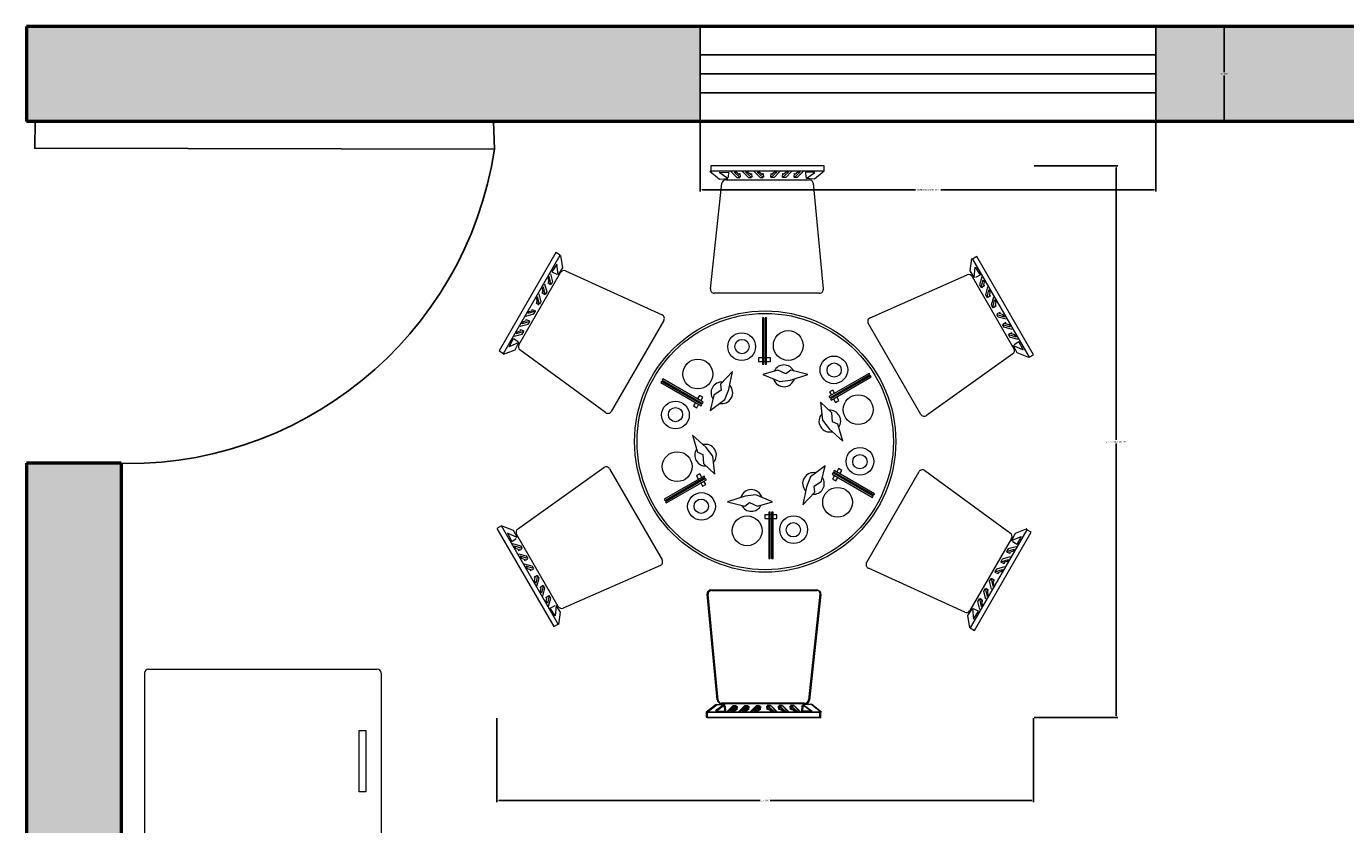
# Model space of a CAD drawing. Units: inches. Extents: x 1771 to 3025, y 319 to 889.
# Tile 8 of 35: x 1800 to 1939, y 805 to 889. Entities that reach past the tile are written whole.
import ezdxf

# ---------------------------------------------------------------- set-up
doc = ezdxf.new("R2010")
doc.units = ezdxf.units.IN
doc.header["$MEASUREMENT"] = 0
for name, color, linetype, lineweight in [('A-ANNO-DIMS', 2, 'Continuous', 18), ('A-DOOR', 4, 'Continuous', 25), ('A-FURN', 8, 'Continuous', 18), ('A-GLAZ', 40, 'Continuous', 25), ('A-WALL', 7, 'Continuous', 50), ('A-WALL-PATT', 254, 'Continuous', 13)]:
    doc.layers.add(name, color=color, linetype=linetype, lineweight=lineweight)
doc.styles.get("Standard").update_dxf_attribs({"font": 'arial.ttf'})
doc.dimstyles.get("Standard").update_dxf_attribs({"dimtxt": 0.18, "dimasz": 0.18, "dimexe": 0.18, "dimexo": 0.0625, "dimgap": 0.09, "dimtad": 0, "dimtih": 1, "dimtoh": 1, "dimdec": 4, "dimzin": 0, "dimdsep": 46, "dimtxsty": 'Standard', "dimcen": 0.09, "dimadec": 0, "dimazin": 0, "dimtfac": 1, "dimtdec": 4, "dimtofl": 0, "dimtmove": 0, "dimatfit": 3, "dimfxl": 1, "dimtolj": 1, "dimtzin": 0, "dimarcsym": 0})

# ---------------------------------------------------------------- blocks, each defined once
blk = doc.blocks.new('A$C1C317F9A')
for p, q in [((0.8756, 2.2462), (0.9155, 2.2143)), ((0.8788, 2.2685), (0.8788, 2.2478)), ((1.3449, 2.2685), (0.8788, 2.2685)), ((0.8788, 2.2478), (1.3449, 2.2478)), ((0.9139, 2.2414), (0.9522, 2.243)), ((0.949, 2.2159), (0.9139, 2.2414)), ((0.9522, 2.243), (0.9506, 2.2206)), ((0.9618, 2.2446), (0.9857, 2.2206)), ((0.9745, 2.243), (0.9841, 2.243)), ((0.9985, 2.2206), (0.9745, 2.243)), ((0.9841, 2.243), (0.9953, 2.2334)), ((0.9953, 2.2334), (0.9985, 2.2366)), ((0.9985, 2.2366), (1.0001, 2.2222)), ((1.0097, 2.2446), (1.0336, 2.2206)), ((1.0224, 2.243), (1.032, 2.243)), ((1.0464, 2.2206), (1.0224, 2.243)), ((1.032, 2.243), (1.0432, 2.2334)), ((1.0432, 2.2334), (1.0464, 2.2366)), ((1.0464, 2.2366), (1.048, 2.2222)), ((1.0576, 2.2446), (1.0815, 2.2206)), ((1.0703, 2.243), (1.0799, 2.243)), ((1.0943, 2.2206), (1.0703, 2.243)), ((1.0799, 2.243), (1.0911, 2.2334)), ((1.0911, 2.2334), (1.0943, 2.2366)), ((1.0943, 2.2366), (1.0959, 2.2222)), ((1.1262, 2.2366), (1.1246, 2.2222)), ((1.1262, 2.2206), (1.1502, 2.243)), ((1.1294, 2.2334), (1.1262, 2.2366)), ((1.1406, 2.243), (1.1294, 2.2334)), ((1.1629, 2.2446), (1.139, 2.2206)), ((1.1502, 2.243), (1.1406, 2.243)), ((1.1741, 2.2366), (1.1725, 2.2222)), ((1.1741, 2.2206), (1.1981, 2.243)), ((1.1773, 2.2334), (1.1741, 2.2366)), ((1.1885, 2.243), (1.1773, 2.2334)), ((1.2108, 2.2446), (1.1869, 2.2206)), ((1.1981, 2.243), (1.1885, 2.243)), ((1.222, 2.2366), (1.2204, 2.2222)), ((1.222, 2.2206), (1.246, 2.243)), ((1.2252, 2.2334), (1.222, 2.2366)), ((1.2364, 2.243), (1.2252, 2.2334)), ((1.2587, 2.2446), (1.2348, 2.2206)), ((1.246, 2.243), (1.2364, 2.243)), ((1.2683, 2.243), (1.2699, 2.2206)), ((1.3066, 2.2414), (1.2683, 2.243)), ((1.2715, 2.2159), (1.3066, 2.2414)), ((1.3449, 2.2462), (1.305, 2.2143)), ((1.3449, 2.2478), (1.3449, 2.2685)), ((0.8775, 1.7628), (0.9251, 2.1968)), ((0.9155, 2.2143), (0.949, 2.2159)), ((0.941, 2.2111), (1.2841, 2.2111)), ((0.9857, 2.2206), (0.9985, 2.2206)), ((1.0336, 2.2206), (1.0464, 2.2206)), ((1.0815, 2.2206), (1.0943, 2.2206)), ((1.139, 2.2206), (1.1262, 2.2206)), ((1.1869, 2.2206), (1.1741, 2.2206)), ((1.2348, 2.2206), (1.222, 2.2206)), ((1.305, 2.2143), (1.2715, 2.2159)), ((1.3, 2.1966), (1.3417, 1.7626)), ((0.2422, 1.9115), (0.0091, 1.5078)), ((0.0271, 1.4974), (0.2602, 1.9011)), ((0.2602, 1.9011), (0.2422, 1.9115)), ((0.2615, 1.9003), (0.2692, 1.8498)), ((0.2465, 1.8648), (0.226, 1.8324)), ((0.2511, 1.8216), (0.2465, 1.8648)), ((0.2692, 1.8498), (0.2511, 1.8216)), ((1.9514, 1.8873), (1.9438, 1.8368)), ((1.9724, 1.8957), (1.9544, 1.8854)), ((1.9544, 1.8854), (2.1875, 1.4816)), ((1.9619, 1.8086), (1.9665, 1.8518)), ((1.9665, 1.8518), (1.987, 1.8194)), ((2.2055, 1.492), (1.9724, 1.8957)), ((0.09, 1.5329), (0.2615, 1.8301)), ((0.2127, 1.7903), (0.2084, 1.7891)), ((0.2148, 1.813), (0.21, 1.8047)), ((0.21, 1.8047), (0.2127, 1.7903)), ((0.2222, 1.7811), (0.2148, 1.813)), ((0.2198, 1.8249), (0.2286, 1.7922)), ((0.2286, 1.7922), (0.2222, 1.7811)), ((0.226, 1.8324), (0.2461, 1.8226)), ((0.282, 1.8367), (0.6787, 1.6557)), ((1.5338, 1.644), (1.9335, 1.8198)), ((1.9438, 1.8368), (1.9619, 1.8086)), ((1.9537, 1.8131), (2.1253, 1.516)), ((1.987, 1.8194), (1.9669, 1.8096)), ((1.9932, 1.8119), (1.9844, 1.7792)), ((1.9908, 1.7681), (1.9982, 1.8)), ((1.9982, 1.8), (2.003, 1.7917)), ((2.003, 1.7917), (2.0003, 1.7773)), ((0.1719, 1.7419), (0.1807, 1.7092)), ((0.1888, 1.7488), (0.1844, 1.7476)), ((0.1844, 1.7476), (0.1961, 1.7391)), ((0.1909, 1.7716), (0.1861, 1.7633)), ((0.1861, 1.7633), (0.1888, 1.7488)), ((0.1982, 1.7396), (0.1909, 1.7716)), ((0.1959, 1.7834), (0.2046, 1.7507)), ((0.2046, 1.7507), (0.1982, 1.7396)), ((0.2084, 1.7891), (0.22, 1.7805)), ((1.3258, 1.7451), (0.8934, 1.7451)), ((1.9844, 1.7792), (1.9908, 1.7681)), ((2.0046, 1.7761), (1.993, 1.7675)), ((2.0003, 1.7773), (2.0046, 1.7761)), ((2.0171, 1.7704), (2.0084, 1.7377)), ((2.0084, 1.7377), (2.0147, 1.7266)), ((2.0147, 1.7266), (2.0221, 1.7585)), ((2.0221, 1.7585), (2.0269, 1.7502)), ((2.0269, 1.7502), (2.0242, 1.7358)), ((2.0242, 1.7358), (2.0286, 1.7346)), ((0.1648, 1.7073), (0.1605, 1.7061)), ((0.1605, 1.7061), (0.1721, 1.6976)), ((0.1669, 1.7301), (0.1621, 1.7218)), ((0.1621, 1.7218), (0.1648, 1.7073)), ((0.1743, 1.6982), (0.1669, 1.7301)), ((0.1807, 1.7092), (0.1743, 1.6982)), ((2.0286, 1.7346), (2.0169, 1.726)), ((2.0411, 1.7289), (2.0323, 1.6962)), ((2.0323, 1.6962), (2.0387, 1.6852)), ((2.0387, 1.6852), (2.0461, 1.7171)), ((2.0525, 1.6931), (2.0409, 1.6846)), ((2.0461, 1.7171), (2.0509, 1.7088)), ((2.0509, 1.7088), (2.0482, 1.6943)), ((2.0482, 1.6943), (2.0525, 1.6931)), ((0.1344, 1.629), (0.1031, 1.6195)), ((0.1031, 1.6195), (0.1078, 1.6278)), ((0.1078, 1.6278), (0.1217, 1.6327)), ((0.1192, 1.6507), (0.1519, 1.6595)), ((0.1217, 1.6327), (0.1206, 1.637)), ((0.1206, 1.637), (0.1338, 1.6312)), ((0.1583, 1.6705), (0.127, 1.6609)), ((0.127, 1.6609), (0.1318, 1.6692)), ((0.128, 1.618), (0.1344, 1.629)), ((0.1318, 1.6692), (0.1457, 1.6741)), ((0.1445, 1.6785), (0.1577, 1.6727)), ((0.1457, 1.6741), (0.1445, 1.6785)), ((0.1519, 1.6595), (0.1583, 1.6705)), ((0.6859, 1.6332), (0.4697, 1.2588)), ((1.091, 1.6437, 0.0908), (1.091, 1.4528, 0.0908)), ((1.097, 1.6437, 0.0908), (1.091, 1.6437, 0.0908)), ((1.097, 1.4528, 0.0908), (1.097, 1.6437, 0.0908)), ((1.1023, 1.6437, 0.0908), (1.1023, 1.4528, 0.0908)), ((1.1083, 1.6437, 0.0908), (1.1023, 1.6437, 0.0908)), ((1.1083, 1.4528, 0.0908), (1.1083, 1.6437, 0.0908)), ((2.0547, 1.6575), (2.086, 1.6479)), ((2.061, 1.6464), (2.0547, 1.6575)), ((2.0685, 1.6655), (2.0552, 1.6597)), ((2.0937, 1.6377), (2.061, 1.6464)), ((2.0673, 1.6611), (2.0685, 1.6655)), ((2.0812, 1.6562), (2.0673, 1.6611)), ((2.086, 1.6479), (2.0812, 1.6562)), ((0.0713, 1.5677), (0.104, 1.5765)), ((0.1104, 1.5876), (0.0791, 1.578)), ((0.0791, 1.578), (0.0839, 1.5863)), ((0.0839, 1.5863), (0.0978, 1.5912)), ((0.0953, 1.6092), (0.128, 1.618)), ((0.0966, 1.5955), (0.1098, 1.5897)), ((0.0978, 1.5912), (0.0966, 1.5955)), ((0.104, 1.5765), (0.1104, 1.5876)), ((1.7426, 1.2469), (1.5264, 1.6214)), ((2.0786, 1.616), (2.1099, 1.6065)), ((2.085, 1.605), (2.0786, 1.616)), ((2.0924, 1.624), (2.0792, 1.6182)), ((2.1177, 1.5962), (2.085, 1.605)), ((2.0913, 1.6196), (2.0924, 1.624)), ((2.1051, 1.6148), (2.0913, 1.6196)), ((2.1026, 1.5745), (2.1339, 1.565)), ((2.1089, 1.5635), (2.1026, 1.5745)), ((2.1164, 1.5825), (2.1031, 1.5767)), ((2.1099, 1.6065), (2.1051, 1.6148)), ((2.1152, 1.5782), (2.1164, 1.5825)), ((2.1291, 1.5733), (2.1152, 1.5782)), ((2.1339, 1.565), (2.1291, 1.5733)), ((0.0502, 1.5246), (0.0679, 1.5586)), ((0.0898, 1.5423), (0.0502, 1.5246)), ((0.0679, 1.5586), (0.0865, 1.5461)), ((0.0745, 1.5125), (0.0898, 1.5423)), ((2.1416, 1.5547), (2.1089, 1.5635)), ((2.1232, 1.5293), (2.1628, 1.5116)), ((2.1385, 1.4995), (2.1232, 1.5293)), ((2.145, 1.5456), (2.1265, 1.5331)), ((2.1628, 1.5116), (2.145, 1.5456)), ((0.0091, 1.5078), (0.0271, 1.4974)), ((0.0269, 1.4939), (0.0745, 1.5125)), ((0.4464, 1.2539), (0.0943, 1.5121)), ((1.0755, 1.4796, 0.0908), (1.0755, 1.4641, 0.0908)), ((1.091, 1.4796, 0.0908), (1.0755, 1.4796, 0.0908)), ((1.1023, 1.4796, 0.0908), (1.097, 1.4796, 0.0908)), ((1.125, 1.4796, 0.0908), (1.1083, 1.4796, 0.0908)), ((1.125, 1.4641, 0.0908), (1.125, 1.4796, 0.0908)), ((2.1208, 1.495), (1.7657, 1.2419)), ((2.1861, 1.4809), (2.1385, 1.4995)), ((2.1875, 1.4816), (2.2055, 1.492)), ((0.9684, 1.4231, 0.0908), (0.9184, 1.3706, 0.0908)), ((0.953, 1.3489, 0.0908), (0.9684, 1.4231, 0.0908)), ((1.0755, 1.4641, 0.0908), (1.091, 1.4641, 0.0908)), ((1.091, 1.4528, 0.0908), (1.097, 1.4528, 0.0908)), ((1.1549, 1.429, 0.0908), (1.0933, 1.4112, 0.0908)), ((1.0933, 1.4112, 0.0908), (1.1623, 1.3815, 0.0908)), ((1.097, 1.4641, 0.0908), (1.1023, 1.4641, 0.0908)), ((1.1023, 1.4528, 0.0908), (1.1083, 1.4528, 0.0908)), ((1.1083, 1.4641, 0.0908), (1.125, 1.4641, 0.0908)), ((1.1882, 1.4134, 0.0908), (1.1549, 1.429, 0.0908)), ((1.2075, 1.4282, 0.0908), (1.1882, 1.4134, 0.0908)), ((1.2061, 1.3874, 0.0908), (1.278, 1.4112, 0.0908)), ((1.278, 1.4112, 0.0908), (1.2075, 1.4282, 0.0908)), ((1.5304, 1.4154, 0.0908), (1.365, 1.3199, 0.0908)), ((1.368, 1.3147, 0.0908), (1.5334, 1.4102, 0.0908)), ((1.5334, 1.4102, 0.0908), (1.5304, 1.4154, 0.0908)), ((0.6765, 1.3825, 0.0908), (0.6735, 1.3774, 0.0908)), ((0.6735, 1.3774, 0.0908), (0.8389, 1.2819, 0.0908)), ((0.8419, 1.2871, 0.0908), (0.6765, 1.3825, 0.0908)), ((0.6822, 1.3924, 0.0908), (0.6792, 1.3872, 0.0908)), ((0.6792, 1.3872, 0.0908), (0.8446, 1.2917, 0.0908)), ((0.8476, 1.2969, 0.0908), (0.6822, 1.3924, 0.0908)), ((0.9184, 1.3706, 0.0908), (0.9216, 1.3464, 0.0908)), ((1.1623, 1.3815, 0.0908), (1.2061, 1.3874, 0.0908)), ((1.5361, 1.4055, 0.0908), (1.3707, 1.3101, 0.0908)), ((1.3737, 1.3049, 0.0908), (1.539, 1.4004, 0.0908)), ((1.539, 1.4004, 0.0908), (1.5361, 1.4055, 0.0908)), ((0.8213, 1.3051, 0.0908), (0.8186, 1.3005, 0.0908)), ((0.8327, 1.3248, 0.0908), (0.8243, 1.3103, 0.0908)), ((0.8461, 1.317, 0.0908), (0.8327, 1.3248, 0.0908)), ((0.8377, 1.3025, 0.0908), (0.8461, 1.317, 0.0908)), ((0.8914, 1.3253, 0.0908), (0.8761, 1.2631, 0.0908)), ((0.8761, 1.2631, 0.0908), (0.9363, 1.308, 0.0908)), ((0.9216, 1.3464, 0.0908), (0.8914, 1.3253, 0.0908)), ((0.9363, 1.308, 0.0908), (0.953, 1.3489, 0.0908)), ((1.365, 1.3199, 0.0908), (1.368, 1.3147, 0.0908)), ((1.3805, 1.3467, 0.0908), (1.3671, 1.339, 0.0908)), ((1.3671, 1.339, 0.0908), (1.3748, 1.3255, 0.0908)), ((1.3707, 1.3101, 0.0908), (1.3737, 1.3049, 0.0908)), ((1.3778, 1.3204, 0.0908), (1.3805, 1.3157, 0.0908)), ((1.3883, 1.3333, 0.0908), (1.3805, 1.3467, 0.0908)), ((1.3835, 1.3106, 0.0908), (1.3918, 1.2961, 0.0908)), ((1.3939, 1.3235, 0.0908), (1.3912, 1.3281, 0.0908)), ((1.3918, 1.2961, 0.0908), (1.4053, 1.3038, 0.0908)), ((1.4053, 1.3038, 0.0908), (1.3969, 1.3183, 0.0908)), ((0.8156, 1.2953, 0.0908), (0.8079, 1.2819, 0.0908)), ((0.8079, 1.2819, 0.0908), (0.8213, 1.2741, 0.0908)), ((0.8213, 1.2741, 0.0908), (0.8291, 1.2876, 0.0908)), ((0.8321, 1.2927, 0.0908), (0.8348, 1.2974, 0.0908)), ((0.8389, 1.2819, 0.0908), (0.8419, 1.2871, 0.0908)), ((0.8446, 1.2917, 0.0908), (0.8476, 1.2969, 0.0908)), ((1.3763, 1.2527, 0.0908), (1.3301, 1.2971, 0.0908)), ((1.3301, 1.2971, 0.0908), (1.3389, 1.2225, 0.0908)), ((1.3795, 1.216, 0.0908), (1.3763, 1.2527, 0.0908)), ((1.3389, 1.2225, 0.0908), (1.366, 1.1876, 0.0908)), ((1.402, 1.2067, 0.0908), (1.3795, 1.216, 0.0908)), ((1.4225, 1.1371, 0.0908), (1.402, 1.2067, 0.0908)), ((0.8033, 1.1609, 0.0908), (0.8238, 1.0913, 0.0908)), ((0.8599, 1.1105, 0.0908), (0.8033, 1.1609, 0.0908)), ((1.366, 1.1876, 0.0908), (1.4225, 1.1371, 0.0908)), ((0.8238, 1.0913, 0.0908), (0.8463, 1.0821, 0.0908)), ((0.8869, 1.0755, 0.0908), (0.8599, 1.1105, 0.0908)), ((0.8463, 1.0821, 0.0908), (0.8495, 1.0454, 0.0908)), ((0.8495, 1.0454, 0.0908), (0.8957, 1.0009, 0.0908)), ((0.8957, 1.0009, 0.0908), (0.8869, 1.0755, 0.0908)), ((1.3498, 1.0349, 0.0908), (1.2896, 0.99, 0.0908)), ((1.3344, 0.9727, 0.0908), (1.3498, 1.0349, 0.0908)), ((0.0847, 0.7751), (0.4398, 1.0281)), ((0.4628, 1.0231), (0.679, 0.6486)), ((0.8522, 0.9931, 0.0908), (0.6868, 0.8977, 0.0908)), ((0.6898, 0.8925, 0.0908), (0.8552, 0.988, 0.0908)), ((0.8578, 0.9833, 0.0908), (0.6925, 0.8878, 0.0908)), ((0.6955, 0.8827, 0.0908), (0.8608, 0.9781, 0.0908)), ((0.834, 1.0019, 0.0908), (0.8206, 0.9942, 0.0908)), ((0.8206, 0.9942, 0.0908), (0.8289, 0.9797, 0.0908)), ((0.8424, 0.9875, 0.0908), (0.834, 1.0019, 0.0908)), ((0.848, 0.9776, 0.0908), (0.8453, 0.9823, 0.0908)), ((0.8552, 0.988, 0.0908), (0.8522, 0.9931, 0.0908)), ((0.8608, 0.9781, 0.0908), (0.8578, 0.9833, 0.0908)), ((1.2896, 0.99, 0.0908), (1.2728, 0.9491, 0.0908)), ((1.3813, 1.0063, 0.0908), (1.3783, 1.0011, 0.0908)), ((1.3783, 1.0011, 0.0908), (1.5437, 0.9057, 0.0908)), ((1.3881, 0.9955, 0.0908), (1.3797, 0.981, 0.0908)), ((1.3797, 0.981, 0.0908), (1.3932, 0.9732, 0.0908)), ((1.5466, 0.9108, 0.0908), (1.3813, 1.0063, 0.0908)), ((1.3869, 1.0161, 0.0908), (1.384, 1.011, 0.0908)), ((1.384, 1.011, 0.0908), (1.5493, 0.9155, 0.0908)), ((1.5523, 0.9207, 0.0908), (1.3869, 1.0161, 0.0908)), ((1.3938, 1.0053, 0.0908), (1.3911, 1.0006, 0.0908)), ((1.3932, 0.9732, 0.0908), (1.4015, 0.9877, 0.0908)), ((1.4045, 1.0239, 0.0908), (1.3968, 1.0105, 0.0908)), ((1.418, 1.0162, 0.0908), (1.4045, 1.0239, 0.0908)), ((1.4045, 0.9929, 0.0908), (1.4072, 0.9975, 0.0908)), ((1.4102, 1.0027, 0.0908), (1.418, 1.0162, 0.0908)), ((1.5196, 0.6368), (1.7358, 1.0113)), ((1.7591, 1.0162), (2.1111, 0.7579)), ((0.8319, 0.9745, 0.0908), (0.8346, 0.9699, 0.0908)), ((0.8376, 0.9647, 0.0908), (0.8453, 0.9513, 0.0908)), ((0.8453, 0.9513, 0.0908), (0.8588, 0.959, 0.0908)), ((0.8588, 0.959, 0.0908), (0.851, 0.9725, 0.0908)), ((1.2728, 0.9491, 0.0908), (1.2574, 0.875, 0.0908)), ((1.2574, 0.875, 0.0908), (1.3074, 0.9275, 0.0908)), ((1.3042, 0.9516, 0.0908), (1.3344, 0.9727, 0.0908)), ((1.3074, 0.9275, 0.0908), (1.3042, 0.9516, 0.0908)), ((0.6868, 0.8977, 0.0908), (0.6898, 0.8925, 0.0908)), ((0.6925, 0.8878, 0.0908), (0.6955, 0.8827, 0.0908)), ((1.0198, 0.9106, 0.0908), (0.9478, 0.8869, 0.0908)), ((0.9478, 0.8869, 0.0908), (1.0183, 0.8698, 0.0908)), ((1.0183, 0.8698, 0.0908), (1.0376, 0.8846, 0.0908)), ((1.0636, 0.9165, 0.0908), (1.0198, 0.9106, 0.0908)), ((1.0376, 0.8846, 0.0908), (1.071, 0.8691, 0.0908)), ((1.1326, 0.8869, 0.0908), (1.0636, 0.9165, 0.0908)), ((1.071, 0.8691, 0.0908), (1.1326, 0.8869, 0.0908)), ((1.5437, 0.9057, 0.0908), (1.5466, 0.9108, 0.0908)), ((1.5493, 0.9155, 0.0908), (1.5523, 0.9207, 0.0908)), ((1.1175, 0.8339, 0.0908), (1.1008, 0.8339, 0.0908)), ((1.1008, 0.8339, 0.0908), (1.1008, 0.8184, 0.0908)), ((1.1008, 0.8184, 0.0908), (1.1175, 0.8184, 0.0908)), ((1.1235, 0.8453, 0.0908), (1.1175, 0.8453, 0.0908)), ((1.1175, 0.8453, 0.0908), (1.1175, 0.6543, 0.0908)), ((1.1235, 0.6543, 0.0908), (1.1235, 0.8453, 0.0908)), ((1.1289, 0.8339, 0.0908), (1.1235, 0.8339, 0.0908)), ((1.1235, 0.8184, 0.0908), (1.1289, 0.8184, 0.0908)), ((1.1349, 0.8453, 0.0908), (1.1289, 0.8453, 0.0908)), ((1.1289, 0.8453, 0.0908), (1.1289, 0.6543, 0.0908)), ((1.1349, 0.6543, 0.0908), (1.1349, 0.8453, 0.0908)), ((1.1504, 0.8339, 0.0908), (1.1349, 0.8339, 0.0908)), ((1.1349, 0.8184, 0.0908), (1.1504, 0.8184, 0.0908)), ((1.1504, 0.8184, 0.0908), (1.1504, 0.8339, 0.0908)), ((0.018, 0.7884), (0, 0.778)), ((0, 0.778), (0.2331, 0.3743)), ((0.2511, 0.3847), (0.018, 0.7884)), ((0.0193, 0.7892), (0.0669, 0.7706)), ((0.0669, 0.7706), (0.0823, 0.7407)), ((2.1784, 0.7726), (1.9453, 0.3689)), ((1.9633, 0.3585), (2.1964, 0.7622)), ((2.1786, 0.7762), (2.131, 0.7576)), ((2.1964, 0.7622), (2.1784, 0.7726)), ((0.0427, 0.7584), (0.0604, 0.7244)), ((0.0823, 0.7407), (0.0427, 0.7584)), ((0.0604, 0.7244), (0.079, 0.737)), ((0.0638, 0.7153), (0.0965, 0.7066)), ((0.2517, 0.4569), (0.0802, 0.7541)), ((0.0965, 0.7066), (0.1029, 0.6955)), ((2.1155, 0.7371), (1.9439, 0.4399)), ((2.131, 0.7576), (2.1156, 0.7277)), ((2.1156, 0.7277), (2.1553, 0.7454)), ((2.1375, 0.7114), (2.119, 0.724)), ((2.1553, 0.7454), (2.1375, 0.7114)), ((0.0716, 0.7051), (0.0764, 0.6968)), ((0.1029, 0.6955), (0.0716, 0.7051)), ((0.0764, 0.6968), (0.0903, 0.6919)), ((0.0878, 0.6738), (0.1205, 0.6651)), ((0.0891, 0.6875), (0.1023, 0.6933)), ((0.0903, 0.6919), (0.0891, 0.6875)), ((0.0955, 0.6636), (0.1003, 0.6553)), ((0.1269, 0.654), (0.0955, 0.6636)), ((0.1003, 0.6553), (0.1142, 0.6504)), ((0.1131, 0.646), (0.1263, 0.6518)), ((0.1205, 0.6651), (0.1269, 0.654)), ((1.1175, 0.6543, 0.0908), (1.1235, 0.6543, 0.0908)), ((1.1289, 0.6543, 0.0908), (1.1349, 0.6543, 0.0908)), ((2.0775, 0.6521), (2.0711, 0.641)), ((2.1102, 0.6608), (2.0775, 0.6521)), ((2.1014, 0.6935), (2.095, 0.6825)), ((2.095, 0.6825), (2.1264, 0.6921)), ((2.1089, 0.6745), (2.0956, 0.6803)), ((2.1341, 0.7023), (2.1014, 0.6935)), ((2.1216, 0.6838), (2.1077, 0.6789)), ((2.1077, 0.6789), (2.1089, 0.6745)), ((2.1264, 0.6921), (2.1216, 0.6838)), ((0.1117, 0.6324), (0.1444, 0.6236)), ((0.1142, 0.6504), (0.1131, 0.646)), ((0.1195, 0.6221), (0.1243, 0.6138)), ((0.1508, 0.6125), (0.1195, 0.6221)), ((0.1243, 0.6138), (0.1382, 0.6089)), ((0.137, 0.6046), (0.1502, 0.6104)), ((0.1382, 0.6089), (0.137, 0.6046)), ((0.1444, 0.6236), (0.1508, 0.6125)), ((0.6716, 0.6261), (0.272, 0.4503)), ((1.9235, 0.4334), (1.5268, 0.6143)), ((2.0535, 0.6106), (2.0471, 0.5995)), ((2.0471, 0.5995), (2.0785, 0.6091)), ((2.061, 0.5915), (2.0477, 0.5973)), ((2.0862, 0.6194), (2.0535, 0.6106)), ((2.0737, 0.6008), (2.0598, 0.5959)), ((2.0711, 0.641), (2.1024, 0.6506)), ((2.0849, 0.633), (2.0717, 0.6388)), ((2.0785, 0.6091), (2.0737, 0.6008)), ((2.0976, 0.6423), (2.0837, 0.6374)), ((2.0837, 0.6374), (2.0849, 0.633)), ((2.1024, 0.6506), (2.0976, 0.6423)), ((0.153, 0.5769), (0.1646, 0.5855)), ((0.1573, 0.5757), (0.153, 0.5769)), ((0.1546, 0.5613), (0.1573, 0.5757)), ((0.1594, 0.553), (0.1546, 0.5613)), ((0.1668, 0.5849), (0.1594, 0.553)), ((0.1644, 0.5411), (0.1732, 0.5738)), ((0.1732, 0.5738), (0.1668, 0.5849)), ((0.1769, 0.5354), (0.1885, 0.544)), ((0.1907, 0.5434), (0.1834, 0.5115)), ((0.1971, 0.5323), (0.1907, 0.5434)), ((2.0248, 0.5608), (2.0312, 0.5719)), ((2.0336, 0.5281), (2.0248, 0.5608)), ((2.0312, 0.5719), (2.0386, 0.54)), ((2.045, 0.5639), (2.0334, 0.5725)), ((2.0386, 0.54), (2.0433, 0.5483)), ((2.0406, 0.5627), (2.045, 0.5639)), ((2.0433, 0.5483), (2.0406, 0.5627)), ((2.0598, 0.5959), (2.061, 0.5915)), ((0.1813, 0.5343), (0.1769, 0.5354)), ((0.1786, 0.5198), (0.1813, 0.5343)), ((0.1834, 0.5115), (0.1786, 0.5198)), ((0.1884, 0.4996), (0.1971, 0.5323)), ((0.2009, 0.4939), (0.2125, 0.5025)), ((0.2052, 0.4928), (0.2009, 0.4939)), ((0.2025, 0.4783), (0.2052, 0.4928)), ((0.2147, 0.5019), (0.2073, 0.47)), ((0.2123, 0.4582), (0.2211, 0.4909)), ((0.2211, 0.4909), (0.2147, 0.5019)), ((0.9055, 0.0734), (0.8638, 0.5074)), ((0.9096, 0.0719), (0.8679, 0.5059)), ((0.8797, 0.5249), (1.3121, 0.5249)), ((0.8838, 0.5234), (1.3162, 0.5234)), ((1.328, 0.5072), (1.2804, 0.0732)), ((1.3321, 0.5057), (1.2845, 0.0717)), ((1.9769, 0.4779), (1.9833, 0.4889)), ((1.9833, 0.4889), (1.9907, 0.457)), ((1.9971, 0.4809), (1.9855, 0.4895)), ((2.0009, 0.5193), (2.0072, 0.5304)), ((2.0096, 0.4866), (2.0009, 0.5193)), ((2.0072, 0.5304), (2.0146, 0.4985)), ((2.0211, 0.5224), (2.0094, 0.531)), ((2.0146, 0.4985), (2.0194, 0.5068)), ((2.0167, 0.5212), (2.0211, 0.5224)), ((2.0194, 0.5068), (2.0167, 0.5212)), ((0.2073, 0.47), (0.2025, 0.4783)), ((0.2185, 0.4507), (0.2386, 0.4604)), ((0.239, 0.4183), (0.2185, 0.4507)), ((0.2436, 0.4615), (0.239, 0.4183)), ((0.2617, 0.4332), (0.2436, 0.4615)), ((1.9363, 0.4202), (1.9544, 0.4484)), ((1.9544, 0.4484), (1.9589, 0.4053)), ((1.9589, 0.4053), (1.9795, 0.4377)), ((1.9795, 0.4377), (1.9593, 0.4474)), ((1.9857, 0.4451), (1.9769, 0.4779)), ((1.9907, 0.457), (1.9955, 0.4653)), ((1.9927, 0.4798), (1.9971, 0.4809)), ((1.9955, 0.4653), (1.9927, 0.4798)), ((0.2331, 0.3743), (0.2511, 0.3847)), ((0.254, 0.3827), (0.2617, 0.4332)), ((1.9439, 0.3697), (1.9363, 0.4202)), ((1.9453, 0.3689), (1.9633, 0.3585)), ((0.8605, 0.0239), (0.9005, 0.0558)), ((0.8647, 0.0223), (0.9046, 0.0543)), ((0.9005, 0.0558), (0.934, 0.0542)), ((0.9046, 0.0543), (0.9381, 0.0527)), ((1.2645, 0.059), (0.9213, 0.059)), ((1.2686, 0.0574), (0.9255, 0.0574)), ((1.29, 0.0558), (1.2565, 0.0542)), ((1.2941, 0.0543), (1.2606, 0.0527)), ((1.3299, 0.0239), (1.29, 0.0558)), ((1.334, 0.0223), (1.2941, 0.0543)), ((0.8605, 0.0223), (0.8605, 0.0015)), ((1.3267, 0.0223), (0.8605, 0.0223)), ((0.8605, 0.0015), (1.3267, 0.0015)), ((0.8647, 0.0207), (0.8647, 0)), ((1.3308, 0.0207), (0.8647, 0.0207)), ((0.8647, 0), (1.3308, 0)), ((0.934, 0.0542), (0.8989, 0.0286)), ((0.8989, 0.0286), (0.9372, 0.027)), ((0.9381, 0.0527), (0.903, 0.0271)), ((0.903, 0.0271), (0.9413, 0.0255)), ((0.9372, 0.027), (0.9356, 0.0494)), ((0.9413, 0.0255), (0.9397, 0.0479)), ((0.9468, 0.0255), (0.9707, 0.0494)), ((0.9509, 0.0239), (0.9748, 0.0479)), ((0.9835, 0.0494), (0.9595, 0.027)), ((0.9595, 0.027), (0.9691, 0.027)), ((0.9876, 0.0479), (0.9636, 0.0255)), ((0.9636, 0.0255), (0.9732, 0.0255)), ((0.9691, 0.027), (0.9803, 0.0366)), ((0.9707, 0.0494), (0.9835, 0.0494)), ((0.9732, 0.0255), (0.9844, 0.0351)), ((0.9748, 0.0479), (0.9876, 0.0479)), ((0.9803, 0.0366), (0.9835, 0.0334)), ((0.9835, 0.0334), (0.9851, 0.0478)), ((0.9844, 0.0351), (0.9876, 0.0319)), ((0.9876, 0.0319), (0.9892, 0.0463)), ((0.9946, 0.0255), (1.0186, 0.0494)), ((0.9988, 0.0239), (1.0227, 0.0479)), ((1.0314, 0.0494), (1.0074, 0.027)), ((1.0074, 0.027), (1.017, 0.027)), ((1.0355, 0.0479), (1.0115, 0.0255)), ((1.0115, 0.0255), (1.0211, 0.0255)), ((1.017, 0.027), (1.0282, 0.0366)), ((1.0186, 0.0494), (1.0314, 0.0494)), ((1.0211, 0.0255), (1.0323, 0.0351)), ((1.0227, 0.0479), (1.0355, 0.0479)), ((1.0282, 0.0366), (1.0314, 0.0334)), ((1.0314, 0.0334), (1.033, 0.0478)), ((1.0323, 0.0351), (1.0355, 0.0319)), ((1.0355, 0.0319), (1.0371, 0.0463)), ((1.0425, 0.0255), (1.0665, 0.0494)), ((1.0467, 0.0239), (1.0706, 0.0479)), ((1.0793, 0.0494), (1.0553, 0.027)), ((1.0553, 0.027), (1.0649, 0.027)), ((1.0834, 0.0479), (1.0594, 0.0255)), ((1.0594, 0.0255), (1.069, 0.0255)), ((1.0649, 0.027), (1.0761, 0.0366)), ((1.0665, 0.0494), (1.0793, 0.0494)), ((1.069, 0.0255), (1.0802, 0.0351)), ((1.0706, 0.0479), (1.0834, 0.0479)), ((1.0761, 0.0366), (1.0793, 0.0334)), ((1.0793, 0.0334), (1.0809, 0.0478)), ((1.0802, 0.0351), (1.0834, 0.0319)), ((1.0834, 0.0319), (1.085, 0.0463)), ((1.1112, 0.0334), (1.1096, 0.0478)), ((1.1112, 0.0494), (1.1351, 0.027)), ((1.124, 0.0494), (1.1112, 0.0494)), ((1.1144, 0.0366), (1.1112, 0.0334)), ((1.1153, 0.0319), (1.1137, 0.0463)), ((1.1256, 0.027), (1.1144, 0.0366)), ((1.1153, 0.0479), (1.1393, 0.0255)), ((1.1281, 0.0479), (1.1153, 0.0479)), ((1.1185, 0.0351), (1.1153, 0.0319)), ((1.1297, 0.0255), (1.1185, 0.0351)), ((1.1479, 0.0255), (1.124, 0.0494)), ((1.1351, 0.027), (1.1256, 0.027)), ((1.152, 0.0239), (1.1281, 0.0479)), ((1.1393, 0.0255), (1.1297, 0.0255)), ((1.1591, 0.0334), (1.1575, 0.0478)), ((1.1591, 0.0494), (1.183, 0.027)), ((1.1719, 0.0494), (1.1591, 0.0494)), ((1.1623, 0.0366), (1.1591, 0.0334)), ((1.1632, 0.0319), (1.1616, 0.0463)), ((1.1735, 0.027), (1.1623, 0.0366)), ((1.1632, 0.0479), (1.1872, 0.0255)), ((1.176, 0.0479), (1.1632, 0.0479)), ((1.1664, 0.0351), (1.1632, 0.0319)), ((1.1776, 0.0255), (1.1664, 0.0351)), ((1.1958, 0.0255), (1.1719, 0.0494)), ((1.183, 0.027), (1.1735, 0.027)), ((1.1999, 0.0239), (1.176, 0.0479)), ((1.1872, 0.0255), (1.1776, 0.0255)), ((1.207, 0.0334), (1.2054, 0.0478)), ((1.207, 0.0494), (1.2309, 0.027)), ((1.2198, 0.0494), (1.207, 0.0494)), ((1.2102, 0.0366), (1.207, 0.0334)), ((1.2111, 0.0319), (1.2095, 0.0463)), ((1.2214, 0.027), (1.2102, 0.0366)), ((1.2111, 0.0479), (1.235, 0.0255)), ((1.2239, 0.0479), (1.2111, 0.0479)), ((1.2143, 0.0351), (1.2111, 0.0319)), ((1.2255, 0.0255), (1.2143, 0.0351)), ((1.2437, 0.0255), (1.2198, 0.0494)), ((1.2309, 0.027), (1.2214, 0.027)), ((1.2478, 0.0239), (1.2239, 0.0479)), ((1.235, 0.0255), (1.2255, 0.0255)), ((1.2533, 0.027), (1.2549, 0.0494)), ((1.2916, 0.0286), (1.2533, 0.027)), ((1.2565, 0.0542), (1.2916, 0.0286)), ((1.2574, 0.0255), (1.259, 0.0479)), ((1.2957, 0.0271), (1.2574, 0.0255)), ((1.2606, 0.0527), (1.2957, 0.0271)), ((1.3267, 0.0015), (1.3267, 0.0223)), ((1.3308, 0), (1.3308, 0.0207))]:
    blk.add_line(p, q)
for centre, radius in [((1.1027, 1.135), 0.537), ((1.1027, 1.135), 0.527), ((1.0059, 1.525, 0.0908), 0.0569), ((1.1975, 1.5297, 0.0908), 0.0613), ((1.0072, 1.5257, 0.0908), 0.0294), ((0.8256, 1.4126, 0.0908), 0.0613), ((1.385, 1.4297, 0.0908), 0.0569), ((1.3863, 1.4289, 0.0908), 0.0294), ((1.4849, 1.2661, 0.0908), 0.0613), ((0.7338, 1.2443, 0.0908), 0.0569), ((0.7339, 1.2458, 0.0908), 0.0294), ((0.741, 1.0319, 0.0908), 0.0613), ((1.4921, 1.0537, 0.0908), 0.0569), ((1.492, 1.0522, 0.0908), 0.0294), ((0.8408, 0.8683, 0.0908), 0.0569), ((1.4003, 0.8854, 0.0908), 0.0613), ((0.8396, 0.8691, 0.0908), 0.0294), ((1.0283, 0.7683, 0.0908), 0.0613), ((1.2199, 0.773, 0.0908), 0.0569), ((1.2186, 0.7723, 0.0908), 0.0294)]:
    blk.add_circle(centre, radius)
for centre, radius, start, end in [((0.941, 2.1951), 0.016, 90, 173.7428), ((1.2841, 2.1951), 0.016, 5.4801, 90), ((0.2754, 1.8222), 0.016, 65.4801, 150), ((1.9399, 1.8052), 0.016, 30, 113.7428), ((0.8934, 1.7611), 0.016, 173.7428, 270), ((1.3258, 1.7611), 0.016, 270, 5.4801), ((0.6721, 1.6412), 0.016, 330, 65.4801), ((1.5403, 1.6294), 0.016, 113.7428, 210), ((0.1038, 1.525), 0.016, 150, 233.7428), ((2.1115, 1.508), 0.016, 305.4801, 30), ((1.1801, 1.4052, 0.0908), 0.0446, 26.6641, 154.1442), ((0.9246, 1.3353, 0.0908), 0.0446, 86.6641, 214.1442), ((0.9246, 1.3353, 0.0908), 0.0446, 257.0611, 44.0662), ((1.1801, 1.4052, 0.0908), 0.0446, 197.0611, 344.0662), ((0.4559, 1.2667), 0.016, 233.7428, 330), ((1.3684, 1.2189, 0.0908), 0.0446, 137.0611, 284.0662), ((1.3684, 1.2189, 0.0908), 0.0446, 326.6641, 94.1442), ((1.7565, 1.2549), 0.016, 210, 305.4801), ((0.8574, 1.0791, 0.0908), 0.0446, 146.6641, 274.1442), ((0.8574, 1.0791, 0.0908), 0.0446, 317.0611, 104.0662), ((0.449, 1.0151), 0.016, 30, 125.4801), ((1.3012, 0.9627, 0.0908), 0.0446, 77.0611, 224.0662), ((1.3012, 0.9627, 0.0908), 0.0446, 266.6641, 34.1442), ((1.7496, 1.0033), 0.016, 53.7428, 150), ((1.0457, 0.8928, 0.0908), 0.0446, 17.0611, 164.0662), ((1.0457, 0.8928, 0.0908), 0.0446, 206.6641, 334.1442), ((0.094, 0.7621), 0.016, 125.4801, 210), ((2.1017, 0.7451), 0.016, 330, 53.7428), ((0.6652, 0.6407), 0.016, 293.7428, 30), ((1.5334, 0.6288), 0.016, 150, 245.4801), ((0.8797, 0.5089), 0.016, 90, 185.4801), ((0.8838, 0.5074), 0.016, 90, 185.4801), ((1.3121, 0.5089), 0.016, 353.7428, 90), ((1.3162, 0.5074), 0.016, 353.7428, 90), ((0.2656, 0.4649), 0.016, 210, 293.7428), ((1.9301, 0.4479), 0.016, 245.4801, 330), ((0.9213, 0.0749), 0.016, 185.4801, 270), ((0.9255, 0.0734), 0.016, 185.4801, 270), ((1.2645, 0.0749), 0.016, 270, 353.7428), ((1.2686, 0.0734), 0.016, 270, 353.7428)]:
    blk.add_arc(centre, radius, start, end)
blk = doc.blocks.new('A$C43BC2F3A')
for p, q in [((0, 1490.5), (0, 93.5)), ((10, 1500), (590, 1500)), ((600, 1490), (600, 93.5)), ((590, 83.5), (10.3, 83.5)), ((22.6, 83.5), (561, 83.5)), ((30.8, 0), (30.8, 83.5)), ((561, 83.5), (561, 0)), ((561, 0), (30.8, 0))]:
    blk.add_line(p, q)
for points in [[(561, 1344.2), (561, 1188.3), (544.3, 1188.3), (544.3, 1344.2)], [(561, 949), (561, 743), (544.3, 743), (544.3, 949)]]:
    blk.add_lwpolyline(points, close=True)
for points in [[(600, 1060.3), (0, 1060.3)], [(600, 1043.6), (0, 1043.6)]]:
    blk.add_lwpolyline(points)
for centre, radius, start, end in [((10, 1490), 10, 90, 180), ((590, 1490), 10, 0, 90), ((10.5, 94), 10.5, 182.8791, 268.8051), ((590, 93.5), 10, 270, 0)]:
    blk.add_arc(centre, radius, start, end)
blk = doc.blocks.new('DOOR-39')
blk.add_lwpolyline([(48.33, 36.05), (48.44, 33.13), (0, 33.22), (0.05, 36.05)], close=True)
blk.add_arc((9.8, 39.1), 39.1, 267.0753, 351.2184)
blk = doc.blocks.new('WIN-48')
for p, q in [((0, 0), (0, 10)), ((48, 0), (48, 10)), ((0, 7), (48, 7)), ((0, 5), (48, 5)), ((0, 3), (48, 3))]:
    blk.add_line(p, q)
blk = doc.blocks.new('*D24')
at = {"layer": 'A-ANNO-DIMS', "color": 0, "lineweight": -2, "transparency": 16777216}
for p, q in [((1870.72, 878.57), (1870.72, 871.25)), ((1918.72, 878.57), (1918.72, 871.25)), ((1870.9, 871.43), (1893.38, 871.43)), ((1918.54, 871.43), (1896.07, 871.43))]:
    blk.add_line(p, q, dxfattribs=at)
at = {"layer": 'A-ANNO-DIMS', "color": 0, "transparency": 16777216}
for points in [[(1870.9, 871.46), (1870.9, 871.4), (1870.72, 871.43)], [(1918.54, 871.46), (1918.54, 871.4), (1918.72, 871.43)]]:
    blk.add_solid(points, dxfattribs=at)
at = {"layer": 'Defpoints', "color": 0, "transparency": 16777216}
for p in [(1870.72, 878.63), (1918.72, 878.63), (1918.72, 871.43)]:
    blk.add_point(p, dxfattribs=at)
at = {"layer": 'A-ANNO-DIMS', "color": 0, "transparency": 16777216, "insert": (1894.72, 871.43), "char_height": 0.18, "attachment_point": 5}
blk.add_mtext('\\A1;WINDOW W1 48 TYP.', dxfattribs=at)
blk = doc.blocks.new('*D25')
at = {"layer": 'A-ANNO-DIMS', "color": 0, "lineweight": -2, "transparency": 16777216}
for p, q in [((1918.79, 888.63), (1926.1, 888.63)), ((1925.92, 888.45), (1925.92, 883.82)), ((1925.92, 878.81), (1925.92, 883.45)), ((1918.79, 878.63), (1926.1, 878.63))]:
    blk.add_line(p, q, dxfattribs=at)
at = {"layer": 'A-ANNO-DIMS', "color": 0, "transparency": 16777216}
for points in [[(1925.89, 888.45), (1925.95, 888.45), (1925.92, 888.63)], [(1925.89, 878.81), (1925.95, 878.81), (1925.92, 878.63)]]:
    blk.add_solid(points, dxfattribs=at)
at = {"layer": 'Defpoints', "color": 0, "transparency": 16777216}
for p in [(1918.72, 888.63), (1925.92, 888.63), (1918.72, 878.63)]:
    blk.add_point(p, dxfattribs=at)
at = {"layer": 'A-ANNO-DIMS', "color": 0, "transparency": 16777216, "insert": (1925.92, 883.63), "char_height": 0.18, "attachment_point": 5}
blk.add_mtext('\\A1;10 TYP.', dxfattribs=at)
blk = doc.blocks.new('*D48')
at = {"layer": 'A-ANNO-DIMS', "color": 0, "lineweight": -2, "transparency": 16777216}
for p, q in [((1905.88, 873.95), (1914.71, 873.95)), ((1914.53, 873.77), (1914.53, 845.07)), ((1914.53, 816), (1914.53, 844.7)), ((1905.88, 815.82), (1914.71, 815.82))]:
    blk.add_line(p, q, dxfattribs=at)
at = {"layer": 'A-ANNO-DIMS', "color": 0, "transparency": 16777216}
for points in [[(1914.5, 873.77), (1914.56, 873.77), (1914.53, 873.95)], [(1914.5, 816), (1914.56, 816), (1914.53, 815.82)]]:
    blk.add_solid(points, dxfattribs=at)
at = {"layer": 'Defpoints', "color": 0, "transparency": 16777216}
for p in [(1905.81, 873.95), (1914.53, 873.95), (1905.81, 815.82)]:
    blk.add_point(p, dxfattribs=at)
at = {"layer": 'A-ANNO-DIMS', "color": 0, "transparency": 16777216, "insert": (1914.53, 844.88), "char_height": 0.18, "attachment_point": 5}
blk.add_mtext('\\A1;DINING SET 58 TYP.', dxfattribs=at)
blk = doc.blocks.new('*D49')
at = {"layer": 'A-ANNO-DIMS', "color": 0, "lineweight": -2, "transparency": 16777216}
for p, q in [((1849.3, 815.76), (1849.3, 806.92)), ((1905.81, 815.76), (1905.81, 806.92)), ((1849.48, 807.1), (1877.03, 807.1)), ((1905.63, 807.1), (1878.09, 807.1))]:
    blk.add_line(p, q, dxfattribs=at)
at = {"layer": 'A-ANNO-DIMS', "color": 0, "transparency": 16777216}
for points in [[(1849.48, 807.13), (1849.48, 807.07), (1849.3, 807.1)], [(1905.63, 807.13), (1905.63, 807.07), (1905.81, 807.1)]]:
    blk.add_solid(points, dxfattribs=at)
at = {"layer": 'Defpoints', "color": 0, "transparency": 16777216}
for p in [(1849.3, 815.82), (1905.81, 815.82), (1905.81, 807.1)]:
    blk.add_point(p, dxfattribs=at)
at = {"layer": 'A-ANNO-DIMS', "color": 0, "transparency": 16777216, "insert": (1877.56, 807.1), "char_height": 0.18, "attachment_point": 5}
blk.add_mtext('\\A1;57 TYP.', dxfattribs=at)

msp = doc.modelspace()

# ---------------------------------------------------------------- hatches: boundary and pattern name
at = {"layer": 'A-WALL-PATT'}
h = msp.add_hatch(color=256, dxfattribs=at)
h.dxf.hatch_style = 1
h.paths.add_polyline_path([(1870.72, 888.63), (1799.72, 888.63), (1799.72, 878.63), (1870.72, 878.63)])
h.paths.add_polyline_path([(1968.77, 888.63), (1918.72, 888.63), (1918.72, 878.63), (1941.72, 878.63), (1941.72, 830.63), (1946.72, 830.63), (1946.72, 878.63), (1968.77, 878.63)])
h.paths.add_polyline_path([(2059.68, 888.63), (2016.77, 888.63), (2016.77, 878.63), (2037.72, 878.63), (2037.72, 794.63), (1941.72, 794.63), (1941.72, 758.63), (1941.72, 664.63), (1946.72, 664.63), (1946.72, 712), (1946.72, 789.63), (2054.72, 789.63), (2054.72, 794.63), (2042.33, 794.63), (2042.33, 798.62), (2042.33, 835.5), (2042.72, 878.63), (2059.68, 878.63)])
h.paths.add_polyline_path([(2100.72, 888.63), (2077.68, 888.63), (2077.68, 878.63), (2090.72, 878.63), (2090.72, 789.63), (2090.72, 768.61), (2100.72, 768.61)])
h.paths.add_polyline_path([(2100.72, 720.61), (2090.72, 720.61), (2090.72, 669.63), (1982.72, 669.63), (1982.72, 664.63), (2001.72, 664.63), (2001.72, 652.63), (2006.72, 652.63), (2006.72, 664.63), (2049.52, 664.63, -0.385549), (2050.52, 664.63), (2090.72, 664.63), (2090.72, 649.17), (2100.72, 649.17)])
edge = h.paths.add_edge_path()
edge.add_line((2100.72, 631.17), (2090.72, 631.17))
edge.add_line((2090.72, 631.17), (2090.72, 616.63))
edge.add_line((2090.72, 616.63), (2001.72, 616.63))
edge.add_line((2001.72, 616.63), (1982.72, 616.63))
edge.add_line((1982.72, 616.63), (1982.72, 611.63))
edge.add_line((1982.72, 611.63), (2024.67, 611.63))
edge.add_spline(control_points=[(2024.67, 611.63), (2027.58, 612.87), (2030.01, 613.31), (2032.47, 613.72)], knot_values=[484.321569, 484.321569, 484.321569, 484.321569, 625.498764, 625.498764, 625.498764, 625.498764], degree=3, periodic=0)
edge.add_line((2032.47, 613.72), (2033.2, 613.72))
edge.add_spline(control_points=[(2033.2, 613.72), (2035.66, 613.31), (2039.46, 612.87), (2042.2, 611.63)], knot_values=[484.321569, 484.321569, 484.321569, 484.321569, 625.498764, 625.498764, 625.498764, 625.498764], degree=3, periodic=0)
edge.add_line((2042.2, 611.63), (2090.72, 611.63))
edge.add_line((2090.72, 611.63), (2090.72, 581.11))
edge.add_line((2090.72, 581.11), (2100.72, 581.11))
edge.add_line((2100.72, 581.11), (2100.72, 631.17))
h.paths.add_polyline_path([(2100.72, 533.11), (2090.72, 533.11), (2090.72, 479.63), (1946.72, 479.63), (1946.72, 616.63), (1936.72, 616.63), (1936.72, 543.63), (1845.72, 543.63), (1845.72, 533.63), (1936.72, 533.63), (1936.72, 469.63), (2090.72, 469.63), (2090.72, 452.76), (2100.72, 452.76)])
h.paths.add_polyline_path([(2100.72, 404.76), (2090.72, 404.76), (2090.72, 393.63), (1936.72, 393.63), (1936.72, 383.63), (2100.72, 383.63)])
h.paths.add_polyline_path([(1905.72, 758.63), (1835.47, 758.63), (1835.47, 758.63), (1813.44, 758.63), (1809.72, 758.63), (1809.72, 842.59, -0.008336), (1808.42, 842.63), (1799.72, 842.63), (1799.72, 690.58), (1809.72, 690.58), (1809.72, 753.63), (1905.72, 753.63)])
h.paths.add_polyline_path([(1809.72, 642.58), (1799.72, 642.58), (1799.72, 533.63), (1809.72, 533.63), (1809.72, 581)])

# ---------------------------------------------------------------- linework, layer by layer
at = {"layer": 'A-WALL'}
for p, q in [((2100.72, 888.63), (1799.72, 888.63)), ((1799.72, 888.63), (1799.72, 878.63)), ((1941.72, 878.63), (1799.72, 878.63)), ((1809.72, 842.63), (1799.72, 842.63)), ((1799.72, 842.63), (1799.72, 533.63)), ((1809.72, 842.63), (1809.72, 758.63))]:
    msp.add_line(p, q, dxfattribs=at)

# ---------------------------------------------------------------- block references
at = {"layer": 'A-DOOR'}
msp.add_blockref('DOOR-39', (1800.61, 842.58), dxfattribs=at)
at = {"layer": 'A-FURN'}
for name, p, xscale, yscale, zscale in [('A$C1C317F9A', (1849.3, 815.82), 25.6235517785217, 25.6235517785217, 25.6235517785217), ('A$C43BC2F3A', (1812.17, 758.63), 0.0415387277892195, 0.0415387277892195, 0.0415387277892195)]:
    msp.add_blockref(name, p, dxfattribs=dict(at, xscale=xscale, yscale=yscale, zscale=zscale))
at = {"layer": 'A-GLAZ'}
msp.add_blockref('WIN-48', (1870.72, 878.63), dxfattribs=at)

# ---------------------------------------------------------------- dimensions: what is measured, and where the dimension line sits
at = {"layer": 'A-ANNO-DIMS'}
for base, p1, p2, text, picture, middle in [((1925.92, 888.63), (1918.72, 878.63), (1918.72, 888.63), '<> TYP.', '*D25', (1925.92, 883.63)), ((1914.53, 873.95), (1905.81, 815.82), (1905.81, 873.95), 'DINING SET <> TYP.', '*D48', (1914.53, 844.88))]:
    dim = msp.add_linear_dim(base=base, p1=p1, p2=p2, angle=90, text=text, dimstyle='Standard', override={"dimdec": 0, "dimrnd": 0, "dimzin": 0, "dimlunit": 2}, dxfattribs=at)
    dim.commit()
    dim.dimension.update_dxf_attribs({"geometry": picture, "text_midpoint": middle})
for base, p1, p2, text, picture, middle in [((1918.72, 871.43), (1870.72, 878.63), (1918.72, 878.63), 'WINDOW W1 <> TYP.', '*D24', (1894.72, 871.43)), ((1905.81, 807.1), (1849.3, 815.82), (1905.81, 815.82), '<> TYP.', '*D49', (1877.56, 807.1))]:
    dim = msp.add_linear_dim(base=base, p1=p1, p2=p2, text=text, dimstyle='Standard', override={"dimdec": 0, "dimrnd": 0, "dimzin": 0, "dimlunit": 2}, dxfattribs=at)
    dim.commit()
    dim.dimension.update_dxf_attribs({"geometry": picture, "text_midpoint": middle})

doc.saveas('drawing.dxf')
